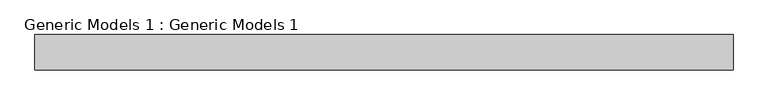
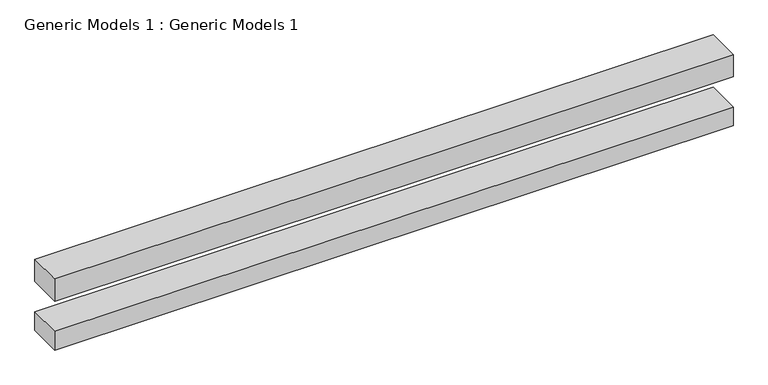
"""IFC4 building model written with IfcOpenShell, lengths in millimetres: proxy geometry, Generic Models 1 : Generic Models 1."""

from ifc_helpers import new_model, si_unit, frame, origin, place, context, project, spatial, polyline, outline, extrude, source, transform, mapped, element, save


def generic_models_1_generic_models_1_a47648ae(model_context):
    return source(origin(), model_context, "Body", "SweptSolid", [
        extrude(outline(polyline([(3942.7077953, -8675.4830082), (-2081.5601778, -8675.4830082), (-2081.5601778, -8370.6830082), (3942.7077953, -8370.6830082), (3942.7077953, -8675.4830082)])), frame((0.0, 0.0, 741.6565496), z_axis=(0.0, 0.0, 1.0), x_axis=(1.0, 0.0, 0.0)), (0.0, 0.0, 1.0), 209.0763108),
        extrude(outline(polyline([(3942.7077953, -8675.4830082), (-2081.5601778, -8675.4830082), (-2081.5601778, -8370.6830082), (3942.7077953, -8370.6830082), (3942.7077953, -8675.4830082)])), frame((0.0, 0.0, 281.315375), z_axis=(0.0, 0.0, 1.0), x_axis=(1.0, 0.0, 0.0)), (0.0, 0.0, 1.0), 175.884625),
    ])


if __name__ == "__main__":
    model = new_model("IFC4")
    model_context = context("Model", 3, world=origin())
    ifc_project = project(units=[si_unit("LENGTHUNIT", "METRE", prefix="MILLI")], contexts=[model_context])
    site = spatial("IfcSite", under=ifc_project)
    building = spatial("IfcBuilding", under=site)
    placement = place(None, origin())
    generic_models_1_generic_models_1_shape = generic_models_1_generic_models_1_a47648ae(model_context)
    element("IfcBuildingElementProxy", 1, Name="Generic Models 1 : Generic Models 1", ObjectType="Generic Models 1 : Generic Models 1", at=placement, inside=building, context=model_context, shape_type="MappedRepresentation", body=[
        mapped(generic_models_1_generic_models_1_shape, transform((0.0, 0.0, 0.0), x_axis=(1.0, 0.0, 0.0), y_axis=(0.0, 1.0, 0.0), z_axis=(0.0, 0.0, 1.0))),
    ])
    save(model, "model.ifc")

# Revit data of these elements
# Element 1 (IfcBuildingElementProxy, "Generic Models 1 : Generic Models 1")
#   Materials on its faces: "Wood - Stained", "Softwood, Lumber"
# Materials
#   "Wood - Stained": class "Wood", colour RGB 224 178 126, transparency 0, Cost = 0
#   "Softwood, Lumber": class "Wood", colour RGB 223 192 134, transparency 0, Description = "Pinus Echinata", Cost = 0
